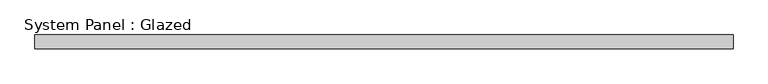
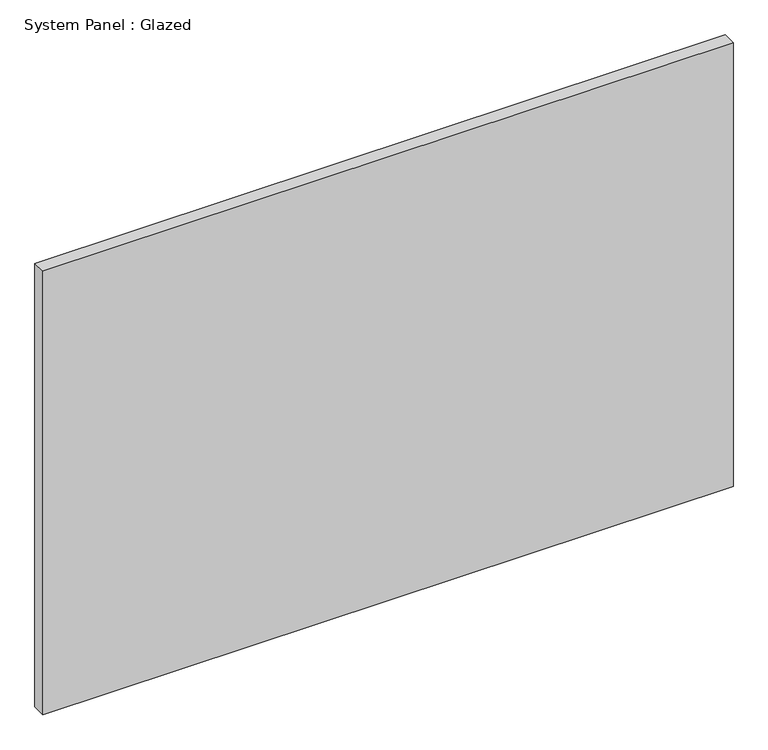
"""IFC4 building model written with IfcOpenShell, lengths in millimetres: plate geometry, System Panel : Glazed."""

from ifc_helpers import new_model, si_unit, origin, origin_with_axes, place, context, project, spatial, polyline, outline, extrude, source, transform, mapped, element, save


def system_panel_glazed_5ee7ee01(model_context):
    return source(origin(), model_context, "Body", "SweptSolid", [
        extrude(outline(polyline([(650.822966, 19.05), (-650.822966, 19.05), (-650.822966, 44.45), (650.822966, 44.45), (650.822966, 19.05)])), origin_with_axes(), (0.0, 0.0, 1.0), 884.8113392),
    ])


if __name__ == "__main__":
    model = new_model("IFC4")
    model_context = context("Model", 3, world=origin())
    ifc_project = project(units=[si_unit("LENGTHUNIT", "METRE", prefix="MILLI")], contexts=[model_context])
    site = spatial("IfcSite", under=ifc_project)
    building = spatial("IfcBuilding", under=site)
    placement = place(None, origin())
    system_panel_glazed_shape = system_panel_glazed_5ee7ee01(model_context)
    element("IfcPlate", 1, ObjectType="System Panel : Glazed", at=placement, inside=building, context=model_context, shape_type="MappedRepresentation", body=[
        mapped(system_panel_glazed_shape, transform((0.0, 0.0, 0.0), x_axis=(1.0, 0.0, 0.0), y_axis=(0.0, 1.0, 0.0), z_axis=(0.0, 0.0, 1.0))),
    ])
    save(model, "model.ifc")

# Revit data of these elements
# Type "System Panel : Glazed"
#   Construction Type Id = "GSP4R"
#   Analytic Construction = "1/8 in Pilkington single glazing"
#   Visual Light Transmittance = 0.9
#   Solar Heat Gain Coefficient = 0.86
#   Heat Transfer Coefficient (U) = 1.18115 BTU/(h·ft²·°F)
#   Define Thermal Properties by = 1
# Element 1 (IfcPlate, "System Panel : Glazed")
#   Materials on its faces: "Glass"
# Materials
#   "Glass": class "Glass", colour RGB 0 128 192, transparency 0.75, Description = "Soda Lime Glass", Cost = 0
